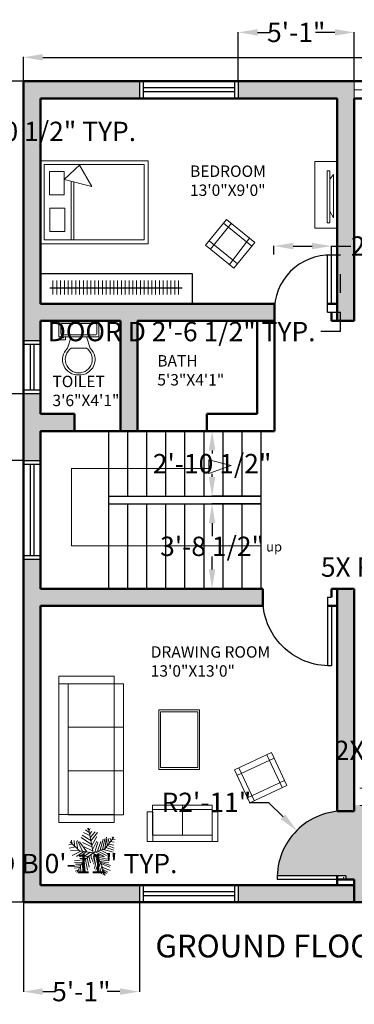
# Model space of a CAD drawing. Units: inches. Extents: x 18 to 9768, y 4 to 3529.
# Tile 4 of 6: x 9249 to 9424, y 3005 to 3523. Entities that reach past the tile are written whole.
import ezdxf

# ---------------------------------------------------------------- set-up
doc = ezdxf.new("R2010")
doc.units = ezdxf.units.IN
doc.header["$MEASUREMENT"] = 0
doc.linetypes.add('ACAD_ISO02W100', pattern=[15, 12, -3])
for name, color, linetype, lineweight in [('A-ANNO-DIMS', 2, 'Continuous', 18), ('A-ANNO-SYMB', 2, 'Continuous', 18), ('A-ANNO-TEXT', 7, 'Continuous', 25), ('A-AREA-IDEN', 7, 'Continuous', 18), ('A-CASE-PATT', 9, 'Continuous', 13), ('A-EQPM', 8, 'Continuous', 18), ('A-FLOR-CASE', 9, 'Continuous', 25), ('A-FLOR-FIXT', 9, 'Continuous', 18), ('A-FLOR-STRS', 7, 'Continuous', 25), ('A-FURN', 8, 'Continuous', 18), ('A-WALL-OVHD', 8, 'ACAD_ISO02W100', 18), ('A-WALL-PATT', 252, 'Continuous', 13), ('L-PLNT', 3, 'Continuous', 18), ('WAL', 7, 'Continuous', 50)]:
    doc.layers.add(name, color=color, linetype=linetype, lineweight=lineweight)
for name, color, linetype, lineweight, true_color in [('A-DOOR', 30, 'Continuous', 25, 0xf8991e), ('A-FLOR-PATT', 254, 'Continuous', 13, 0xddb3d4), ('A-GLAZ', 177, 'Continuous', 25, 0x293189)]:
    doc.layers.add(name, color=color, linetype=linetype, lineweight=lineweight, true_color=true_color)
doc.styles.get("Standard").update_dxf_attribs({"font": 'arial.ttf'})
doc.dimstyles.get("Standard").update_dxf_attribs({"dimtxt": 10.18, "dimasz": 10.18, "dimexe": 0.18, "dimexo": 0.0625, "dimgap": 0.09, "dimtad": 0, "dimtih": 1, "dimtoh": 1, "dimdec": 0, "dimzin": 0, "dimdsep": 46, "dimlunit": 3, "dimtxsty": 'Standard', "dimcen": 0.09, "dimadec": 0, "dimazin": 0, "dimtfac": 1, "dimtdec": 0, "dimtofl": 0, "dimtmove": 0, "dimatfit": 3, "dimfxl": 1, "dimtolj": 1, "dimtzin": 0, "dimarcsym": 0})

# ---------------------------------------------------------------- blocks, each defined once
blk = doc.blocks.new('*U2')
for p, q in [((9.5, -6), (9.5, -2)), ((-10, -8.5), (-8, -8.5)), ((-10, -9.5), (-10, -8.5)), ((-7, -9.5), (-10, -9.5)), ((-8, -8.5), (-8, -8)), ((-7, -8), (-7, -9.5)), ((-4, -8), (-6, -14)), ((4, -8), (6, -14)), ((4, -14), (-4, -14))]:
    blk.add_line(p, q)
blk.add_lwpolyline([(10.5, -8), (10.5, 0), (-10.5, 0), (-10.5, -8)], close=True)
for points in [[(-9.5, -2), (-9.5, -6)], [(8.5, -1), (-8.5, -1)], [(-8.5, -7), (8.5, -7)]]:
    blk.add_lwpolyline(points)
for centre, radius, start, end in [((-8.625, -1.875), 0.8839, 81.8699, 188.1301), ((8.625, -1.875), 0.8839, 351.8699, 98.1301), ((-8.625, -6.125), 0.8839, 171.869898, 278.1301), ((8.625, -6.125), 0.8839, 261.8699, 8.1301), ((-0.4772, -19.9188), 8.0953, 133.01722, 273.38), ((0.0374, -19.8731), 7.127, 124.50543, 269.7), ((-0.0373, -19.8731), 7.127, 270.3, 55.4946), ((0.4773, -19.9188), 8.0953, 266.62, 46.9828)]:
    blk.add_arc(centre, radius, start, end)
blk = doc.blocks.new('*U6')
for p, q in [((-7.288, 39.707), (-21.778, 46.673)), ((-8.737, 47.138), (-17.069, 52.711)), ((-10.186, 53.64), (-13.084, 55.962)), ((0, 0), (-10.5, 57)), ((-9.099, 51.782), (-6.563, 55.962)), ((-7.65, 43.423), (-2.578, 49.46)), ((-5.839, 35.992), (4.667, 48.067)), ((-5.114, 27.632), (10.463, 46.673)), ((-31.5, 4.5), (-52.5, 25.5)), ((-48.585, 21.131), (-49.309, 29.026)), ((-43.513, 28.561), (-42.427, 15.558)), ((-38.442, 26.239), (-34.819, 7.663)), ((-35.544, 28.097), (-24.314, 3.947)), ((-14.533, 2.09), (-30.834, 25.31)), ((-3.665, 19.273), (-27.574, 35.527)), ((-5.114, 28.097), (-24.676, 40.636)), ((-24.314, 23.917), (-2.941, 13.7)), ((-2.941, 16.486), (8.652, 37.85)), ((-1.129, 6.734), (9.014, 26.704)), ((3.942, 1.625), (11.187, 24.381)), ((10.101, 3.483), (17.708, 26.239)), ((16.259, 5.805), (23.142, 31.348)), ((22.055, 7.198), (27.489, 32.277)), ((27, 9), (48, 36)), ((27.127, 9.056), (31.112, 35.992)), ((31.836, 30.883), (32.561, 16.486)), ((35.096, 32.741), (37.27, 22.524)), ((38.719, 34.134), (41.979, 28.561)), ((40.53, 25.775), (48.862, 24.846)), ((43.791, 29.954), (51.036, 30.883)), ((44.153, 36.456), (45.239, 32.741)), ((-47.498, 19.737), (-55.83, 18.344)), ((-40.615, 13.7), (-55.105, 10.913)), ((-33.37, 6.269), (-52.207, 5.34)), ((-28.299, 3.483), (-47.86, -5.805)), ((-21.416, 3.018), (-38.079, -8.128)), ((0, 0), (-31.5, 4.5)), ((-15.982, 2.09), (-30.11, -9.521)), ((0, 0), (-22.5, -19.5)), ((-6.563, 1.161), (-21.416, -8.128)), ((-20.691, 13.7), (-1.129, 4.876)), ((0, 0), (27, 9)), ((0, 0), (18, -22.5)), ((6.478, 1.625), (26.04, -8.592)), ((11.187, 3.483), (30.749, -5.805)), ((18.07, 5.805), (35.096, -3.483)), ((24.229, 7.663), (46.688, 1.625)), ((29.662, 12.307), (48.137, 6.269)), ((33.285, 16.486), (48.862, 10.913)), ((36.183, 19.737), (48.137, 17.88)), ((-17.431, -15.094), (-42.789, -18.809)), ((-24.314, -21.596), (-42.427, -22.06)), ((-22.5, -19.5), (-37.5, -45)), ((-15.257, -12.772), (-30.11, -12.772)), ((-20.691, -18.345), (-17.793, -44.352)), ((-6.563, -5.805), (-19.967, -9.985)), ((-17.069, -15.094), (-12.721, -40.172)), ((-13.446, -11.378), (-8.737, -32.741)), ((-9.461, -8.592), (-6.201, -23.453)), ((-4.752, -3.483), (-3.665, -14.629)), ((2.493, -3.019), (-1.491, -20.202)), ((1.769, -2.555), (24.229, -9.521)), ((5.029, -6.27), (2.131, -25.775)), ((9.014, -11.378), (3.58, -35.992)), ((14.085, -16.951), (6.478, -40.172)), ((7.565, -9.056), (32.198, -14.629)), ((18.07, -22.524), (8.289, -45.745)), ((12.274, -15.094), (36.907, -18.809)), ((16.259, -19.738), (36.183, -22.989)), ((18, -22.5), (27, -52.5)), ((18.433, -22.524), (40.53, -29.026)), ((-28.299, -29.026), (-42.789, -31.348)), ((-30.834, -34.135), (-42.427, -35.528)), ((-34.457, -39.708), (-40.978, -42.494)), ((-26.849, -26.24), (-40.253, -25.775)), ((-32.646, -36.921), (-31.921, -44.352)), ((-29.023, -30.884), (-27.936, -43.887)), ((-25.038, -23.918), (-22.865, -45.281)), ((20.244, -30.419), (15.897, -44.816)), ((19.157, -25.311), (38.719, -33.206)), ((22.78, -37.85), (19.519, -48.532)), ((21.331, -32.741), (39.081, -40.636)), ((22.78, -38.314), (34.372, -44.816)), ((24.591, -43.423), (30.749, -47.603)), ((24.591, -45.745), (23.142, -50.854)), ((26.764, -49.925), (28.213, -50.854))]:
    blk.add_line(p, q)
blk = doc.blocks.new('*D7')
at = {"layer": 'A-ANNO-DIMS', "color": 0, "lineweight": -2, "transparency": 16777216}
for p, q in [((9250.43, 3490.42), (9250.43, 3503.16)), ((9260.61, 3502.98), (9433.71, 3502.98)), ((9624.25, 3502.98), (9451.16, 3502.98)), ((9634.43, 3490.42), (9634.43, 3503.16))]:
    blk.add_line(p, q, dxfattribs=at)
at = {"layer": 'A-ANNO-DIMS', "color": 0, "transparency": 16777216}
for points in [[(9260.61, 3504.67), (9260.61, 3501.28), (9250.43, 3502.98)], [(9624.25, 3504.67), (9624.25, 3501.28), (9634.43, 3502.98)]]:
    blk.add_solid(points, dxfattribs=at)
at = {"layer": 'Defpoints', "color": 0, "transparency": 16777216}
for p in [(9634.43, 3502.98), (9250.43, 3490.36), (9634.43, 3490.36)]:
    blk.add_point(p, dxfattribs=at)
at = {"layer": 'A-ANNO-DIMS', "color": 0, "transparency": 16777216, "insert": (9442.43, 3502.98), "char_height": 10.18, "attachment_point": 5}
blk.add_mtext("\\A1;32'", dxfattribs=at)
blk = doc.blocks.new('*D8')
at = {"layer": 'A-ANNO-DIMS', "color": 0, "lineweight": -2, "transparency": 16777216}
for p, q in [((9250.37, 3490.36), (9231.16, 3490.36)), ((9231.34, 3480.18), (9231.34, 3279.65)), ((9231.34, 3068.54), (9231.34, 3269.07)), ((9250.37, 3058.36), (9231.16, 3058.36))]:
    blk.add_line(p, q, dxfattribs=at)
at = {"layer": 'A-ANNO-DIMS', "color": 0, "transparency": 16777216}
for points in [[(9229.65, 3480.18), (9233.04, 3480.18), (9231.34, 3490.36)], [(9229.65, 3068.54), (9233.04, 3068.54), (9231.34, 3058.36)]]:
    blk.add_solid(points, dxfattribs=at)
at = {"layer": 'Defpoints', "color": 0, "transparency": 16777216}
for p in [(9250.43, 3490.36), (9231.34, 3058.36), (9250.43, 3058.36)]:
    blk.add_point(p, dxfattribs=at)
at = {"layer": 'A-ANNO-DIMS', "color": 0, "transparency": 16777216, "insert": (9231.34, 3274.36), "char_height": 10.18, "attachment_point": 5}
blk.add_mtext("\\A1;36'", dxfattribs=at)
blk = doc.blocks.new('WINDOW-48')
for p, q in [((0, 0), (0, 9)), ((2, 0), (2, 9)), ((2, 5.5), (50, 5.5)), ((50, 0), (50, 9)), ((52, 0), (52, 9)), ((2, 3.5), (50, 3.5))]:
    blk.add_line(p, q)
blk = doc.blocks.new('WINDOW-24')
for p, q in [((9, 28), (0, 28)), ((9, 26), (0, 26)), ((3.5, 26), (3.5, 2)), ((5.5, 26), (5.5, 2)), ((9, 2), (0, 2)), ((9, 0), (0, 0))]:
    blk.add_line(p, q)
blk = doc.blocks.new('DOOR-36-W9')
for p, q in [((2, 36.01), (0, 36.01)), ((0, 31.51), (0, 0.01)), ((2, 36.01), (2, 0.01))]:
    blk.add_line(p, q)
blk.add_arc((1, 35.01), 35.01, 268.3634, 1.6366)
blk = doc.blocks.new('DOOR-30-W9')
for p, q in [((25.52, 30.02), (0.02, 30.02)), ((30.02, 28.02), (0.02, 28.02)), ((30.02, 28.02), (30.02, 30.02))]:
    blk.add_line(p, q)
blk.add_arc((29.02, 29.02), 29.02, 178.0251, 271.9749)
blk = doc.blocks.new('*D35')
at = {"layer": 'A-ANNO-DIMS', "color": 0, "lineweight": -2, "transparency": 16777216}
for p, q in [((9412.5, 3399.14), (9417.16, 3399.14)), ((9416.98, 3388.96), (9416.98, 3379.04)), ((9412.5, 3368.86), (9417.16, 3368.86)), ((9416.98, 3368.86), (9416.98, 3358.68)), ((9416.98, 3358.68), (9406.8, 3358.68))]:
    blk.add_line(p, q, dxfattribs=at)
at = {"layer": 'A-ANNO-DIMS', "color": 0, "transparency": 16777216}
for points in [[(9415.28, 3388.96), (9418.67, 3388.96), (9416.98, 3399.14)], [(9415.28, 3379.04), (9418.67, 3379.04), (9416.98, 3368.86)]]:
    blk.add_solid(points, dxfattribs=at)
at = {"layer": 'Defpoints', "color": 0, "transparency": 16777216}
for p in [(9412.43, 3399.14), (9412.43, 3368.86), (9416.98, 3368.86)]:
    blk.add_point(p, dxfattribs=at)
at = {"layer": 'A-ANNO-DIMS', "color": 0, "transparency": 16777216, "insert": (9333.65, 3358.68), "char_height": 10.18, "attachment_point": 5}
blk.add_mtext('\\A1;DOOR D 2\'-6 1/2" TYP.', dxfattribs=at)
blk = doc.blocks.new('*D36')
at = {"layer": 'A-ANNO-DIMS', "color": 0, "lineweight": -2, "transparency": 16777216}
for p, q in [((9382.16, 3399.2), (9382.16, 3403.86)), ((9392.34, 3403.68), (9402.25, 3403.68)), ((9412.43, 3399.2), (9412.43, 3403.86)), ((9412.43, 3403.68), (9422.61, 3403.68))]:
    blk.add_line(p, q, dxfattribs=at)
at = {"layer": 'A-ANNO-DIMS', "color": 0, "transparency": 16777216}
for points in [[(9392.34, 3405.38), (9392.34, 3401.98), (9382.16, 3403.68)], [(9402.25, 3405.38), (9402.25, 3401.98), (9412.43, 3403.68)]]:
    blk.add_solid(points, dxfattribs=at)
at = {"layer": 'Defpoints', "color": 0, "transparency": 16777216}
for p in [(9382.16, 3399.14), (9412.43, 3403.68), (9412.43, 3399.14)]:
    blk.add_point(p, dxfattribs=at)
at = {"layer": 'A-ANNO-DIMS', "color": 0, "transparency": 16777216, "insert": (9465.68, 3403.68), "char_height": 10.18, "attachment_point": 5}
blk.add_mtext('\\A1;2\'-6 1/2" TYP.', dxfattribs=at)
blk = doc.blocks.new('*D49')
at = {"layer": 'A-ANNO-DIMS', "color": 0, "lineweight": -2, "transparency": 16777216}
for p, q in [((9121.17, 3464.01), (9110.99, 3464.01)), ((9131.35, 3465.54), (9131.35, 3463.83)), ((9141.99, 3465.54), (9141.99, 3463.83)), ((9152.17, 3464.01), (9162.35, 3464.01))]:
    blk.add_line(p, q, dxfattribs=at)
at = {"layer": 'A-ANNO-DIMS', "color": 0, "transparency": 16777216}
for points in [[(9121.17, 3465.71), (9121.17, 3462.32), (9131.35, 3464.01)], [(9152.17, 3465.71), (9152.17, 3462.32), (9141.99, 3464.01)]]:
    blk.add_solid(points, dxfattribs=at)
at = {"layer": 'Defpoints', "color": 0, "transparency": 16777216}
for p in [(9131.35, 3465.61), (9141.99, 3465.61), (9141.99, 3464.01)]:
    blk.add_point(p, dxfattribs=at)
at = {"layer": 'A-ANNO-DIMS', "color": 0, "transparency": 16777216, "insert": (9237.11, 3464.01), "char_height": 10.18, "attachment_point": 5}
blk.add_mtext('\\A1;LAMP B 0\'-10 1/2" TYP.', dxfattribs=at)
blk = doc.blocks.new('*D55')
at = {"layer": 'A-ANNO-DIMS', "color": 0, "lineweight": -2, "transparency": 16777216}
for p, q in [((9114.26, 3078.78), (9104.08, 3078.78)), ((9124.44, 3080.36), (9124.44, 3078.6)), ((9135.38, 3080.36), (9135.38, 3078.6)), ((9145.56, 3078.78), (9155.74, 3078.78))]:
    blk.add_line(p, q, dxfattribs=at)
at = {"layer": 'A-ANNO-DIMS', "color": 0, "transparency": 16777216}
for points in [[(9114.26, 3080.48), (9114.26, 3077.09), (9124.44, 3078.78)], [(9145.56, 3080.48), (9145.56, 3077.09), (9135.38, 3078.78)]]:
    blk.add_solid(points, dxfattribs=at)
at = {"layer": 'Defpoints', "color": 0, "transparency": 16777216}
for p in [(9124.44, 3080.42), (9135.38, 3080.42), (9135.38, 3078.78)]:
    blk.add_point(p, dxfattribs=at)
at = {"layer": 'A-ANNO-DIMS', "color": 0, "transparency": 16777216, "insert": (9245.48, 3078.78), "char_height": 10.18, "attachment_point": 5}
blk.add_mtext('\\A1;NIGHTSTAND B 0\'-11" TYP.', dxfattribs=at)
blk = doc.blocks.new('*D63')
at = {"layer": 'A-ANNO-DIMS', "color": 0, "lineweight": -2, "transparency": 16777216}
for p, q in [((9375.37, 3306.36), (9349.5, 3306.36)), ((9349.68, 3296.18), (9349.68, 3294.53)), ((9349.68, 3282.18), (9349.68, 3283.83)), ((9375.37, 3272), (9349.5, 3272))]:
    blk.add_line(p, q, dxfattribs=at)
at = {"layer": 'A-ANNO-DIMS', "color": 0, "transparency": 16777216}
for points in [[(9347.99, 3296.18), (9351.38, 3296.18), (9349.68, 3306.36)], [(9347.99, 3282.18), (9351.38, 3282.18), (9349.68, 3272)]]:
    blk.add_solid(points, dxfattribs=at)
at = {"layer": 'Defpoints', "color": 0, "transparency": 16777216}
for p in [(9349.68, 3306.36), (9375.43, 3306.36), (9375.43, 3272)]:
    blk.add_point(p, dxfattribs=at)
at = {"layer": 'A-ANNO-DIMS', "color": 0, "transparency": 16777216, "insert": (9349.68, 3289.18), "char_height": 10.18, "attachment_point": 5}
blk.add_mtext('\\A1;2\'-10 1/2"', dxfattribs=at)
blk = doc.blocks.new('*D64')
at = {"layer": 'A-ANNO-DIMS', "color": 0, "lineweight": -2, "transparency": 16777216}
for p, q in [((9375.37, 3268), (9349.5, 3268)), ((9349.68, 3257.82), (9349.68, 3251.04)), ((9349.68, 3233.54), (9349.68, 3240.32)), ((9375.37, 3223.36), (9349.5, 3223.36))]:
    blk.add_line(p, q, dxfattribs=at)
at = {"layer": 'A-ANNO-DIMS', "color": 0, "transparency": 16777216}
for points in [[(9347.99, 3257.82), (9351.38, 3257.82), (9349.68, 3268)], [(9347.99, 3233.54), (9351.38, 3233.54), (9349.68, 3223.36)]]:
    blk.add_solid(points, dxfattribs=at)
at = {"layer": 'Defpoints', "color": 0, "transparency": 16777216}
for p in [(9349.68, 3268), (9375.43, 3268), (9375.43, 3223.36)]:
    blk.add_point(p, dxfattribs=at)
at = {"layer": 'A-ANNO-DIMS', "color": 0, "transparency": 16777216, "insert": (9349.68, 3245.68), "char_height": 10.18, "attachment_point": 5}
blk.add_mtext('\\A1;3\'-8 1/2"', dxfattribs=at)
blk = doc.blocks.new('*D65')
at = {"layer": 'A-ANNO-DIMS', "color": 0, "lineweight": -2, "transparency": 16777216}
for p, q in [((9250.43, 3058.3), (9250.43, 3011.2)), ((9311.43, 3058.3), (9311.43, 3011.2)), ((9260.61, 3011.38), (9267.31, 3011.38)), ((9301.25, 3011.38), (9294.55, 3011.38))]:
    blk.add_line(p, q, dxfattribs=at)
at = {"layer": 'A-ANNO-DIMS', "color": 0, "transparency": 16777216}
for points in [[(9260.61, 3013.08), (9260.61, 3009.68), (9250.43, 3011.38)], [(9301.25, 3013.08), (9301.25, 3009.68), (9311.43, 3011.38)]]:
    blk.add_solid(points, dxfattribs=at)
at = {"layer": 'Defpoints', "color": 0, "transparency": 16777216}
for p in [(9250.43, 3058.36), (9311.43, 3058.36), (9311.43, 3011.38)]:
    blk.add_point(p, dxfattribs=at)
at = {"layer": 'A-ANNO-DIMS', "color": 0, "transparency": 16777216, "insert": (9280.93, 3011.38), "char_height": 10.18, "attachment_point": 5}
blk.add_mtext('\\A1;5\'-1"', dxfattribs=at)
blk = doc.blocks.new('*D72')
at = {"layer": 'A-ANNO-DIMS', "color": 0, "lineweight": -2, "transparency": 16777216}
for p, q in [((9414.25, 3516.11), (9404.07, 3516.11)), ((9424.43, 3490.42), (9424.43, 3516.29)), ((9472.43, 3490.42), (9472.43, 3516.29)), ((9482.61, 3516.11), (9492.79, 3516.11))]:
    blk.add_line(p, q, dxfattribs=at)
at = {"layer": 'A-ANNO-DIMS', "color": 0, "transparency": 16777216}
for points in [[(9414.25, 3517.81), (9414.25, 3514.41), (9424.43, 3516.11)], [(9482.61, 3517.81), (9482.61, 3514.41), (9472.43, 3516.11)]]:
    blk.add_solid(points, dxfattribs=at)
at = {"layer": 'Defpoints', "color": 0, "transparency": 16777216}
for p in [(9472.43, 3516.11), (9424.43, 3490.36), (9472.43, 3490.36)]:
    blk.add_point(p, dxfattribs=at)
at = {"layer": 'A-ANNO-DIMS', "color": 0, "transparency": 16777216, "insert": (9448.43, 3516.11), "char_height": 10.18, "attachment_point": 5}
blk.add_mtext('\\A1;4\'-0"', dxfattribs=at)
blk = doc.blocks.new('*D73')
at = {"layer": 'A-ANNO-DIMS', "color": 0, "lineweight": -2, "transparency": 16777216}
for p, q in [((9363.42, 3490.42), (9363.42, 3516.29)), ((9373.6, 3516.11), (9380.31, 3516.11)), ((9414.25, 3516.11), (9407.55, 3516.11)), ((9424.43, 3490.42), (9424.43, 3516.29))]:
    blk.add_line(p, q, dxfattribs=at)
at = {"layer": 'A-ANNO-DIMS', "color": 0, "transparency": 16777216}
for points in [[(9373.6, 3517.81), (9373.6, 3514.41), (9363.42, 3516.11)], [(9414.25, 3517.81), (9414.25, 3514.41), (9424.43, 3516.11)]]:
    blk.add_solid(points, dxfattribs=at)
at = {"layer": 'Defpoints', "color": 0, "transparency": 16777216}
for p in [(9424.43, 3516.11), (9363.42, 3490.36), (9424.43, 3490.36)]:
    blk.add_point(p, dxfattribs=at)
at = {"layer": 'A-ANNO-DIMS', "color": 0, "transparency": 16777216, "insert": (9393.93, 3516.11), "char_height": 10.18, "attachment_point": 5}
blk.add_mtext('\\A1;5\'-1"', dxfattribs=at)
blk = doc.blocks.new('*D78')
at = {"layer": 'A-ANNO-DIMS', "color": 0, "lineweight": -2, "transparency": 16777216}
for p, q in [((9250.37, 3325.86), (9224.5, 3325.86)), ((9224.68, 3315.68), (9224.68, 3313.56)), ((9224.68, 3301.04), (9224.68, 3303.16)), ((9250.37, 3290.86), (9224.5, 3290.86))]:
    blk.add_line(p, q, dxfattribs=at)
at = {"layer": 'A-ANNO-DIMS', "color": 0, "transparency": 16777216}
for points in [[(9222.99, 3315.68), (9226.38, 3315.68), (9224.68, 3325.86)], [(9222.99, 3301.04), (9226.38, 3301.04), (9224.68, 3290.86)]]:
    blk.add_solid(points, dxfattribs=at)
at = {"layer": 'Defpoints', "color": 0, "transparency": 16777216}
for p in [(9224.68, 3325.86), (9250.43, 3325.86), (9250.43, 3290.86)]:
    blk.add_point(p, dxfattribs=at)
at = {"layer": 'A-ANNO-DIMS', "color": 0, "transparency": 16777216, "insert": (9224.68, 3308.36), "char_height": 10.18, "attachment_point": 5}
blk.add_mtext('\\A1;2\'-11"', dxfattribs=at)
blk = doc.blocks.new('*D82')
at = {"layer": 'A-ANNO-DIMS', "color": 0, "lineweight": -2, "transparency": 16777216}
for p, q in [((9517.84, 3173.21), (9518.02, 3173.21)), ((9517.93, 3173.12), (9517.93, 3173.3)), ((9483.02, 3138.3), (9490.22, 3145.5)), ((9472.84, 3138.3), (9483.02, 3138.3))]:
    blk.add_line(p, q, dxfattribs=at)
at = {"layer": 'A-ANNO-DIMS', "color": 0, "transparency": 16777216}
blk.add_solid([(9489.02, 3146.7), (9491.42, 3144.3), (9497.42, 3152.7)], dxfattribs=at)
at = {"layer": 'Defpoints', "color": 0, "transparency": 16777216}
for p in [(9517.93, 3173.21), (9497.42, 3152.7)]:
    blk.add_point(p, dxfattribs=at)
at = {"layer": 'A-ANNO-DIMS', "color": 0, "transparency": 16777216, "insert": (9443.32, 3138.3), "char_height": 10.18, "attachment_point": 5}
blk.add_mtext('\\A1;2X R2\'-5"', dxfattribs=at)
blk = doc.blocks.new('*D84')
at = {"layer": 'A-ANNO-DIMS', "color": 0, "lineweight": -2, "transparency": 16777216}
for p, q in [((9499.78, 3262.71), (9499.96, 3262.71)), ((9499.87, 3262.62), (9499.87, 3262.8)), ((9499.49, 3234.76), (9499.63, 3244.93)), ((9489.31, 3234.76), (9499.49, 3234.76))]:
    blk.add_line(p, q, dxfattribs=at)
at = {"layer": 'A-ANNO-DIMS', "color": 0, "transparency": 16777216}
blk.add_solid([(9497.93, 3244.96), (9501.32, 3244.91), (9499.77, 3255.11)], dxfattribs=at)
at = {"layer": 'Defpoints', "color": 0, "transparency": 16777216}
for p in [(9499.87, 3262.71), (9499.77, 3255.11)]:
    blk.add_point(p, dxfattribs=at)
at = {"layer": 'A-ANNO-DIMS', "color": 0, "transparency": 16777216, "insert": (9448.02, 3234.76), "char_height": 10.18, "attachment_point": 5}
blk.add_mtext('\\A1;5X R0\'-7 1/2"', dxfattribs=at)
blk = doc.blocks.new('*D87')
at = {"layer": 'A-ANNO-DIMS', "color": 0, "lineweight": -2, "transparency": 16777216}
for p, q in [((9369.14, 3110.97), (9379.32, 3110.97)), ((9379.32, 3110.97), (9386.98, 3103.32)), ((9418.84, 3071.36), (9419.02, 3071.36)), ((9418.93, 3071.27), (9418.93, 3071.45))]:
    blk.add_line(p, q, dxfattribs=at)
at = {"layer": 'A-ANNO-DIMS', "color": 0, "transparency": 16777216}
blk.add_solid([(9388.18, 3104.52), (9385.78, 3102.12), (9394.17, 3096.12)], dxfattribs=at)
at = {"layer": 'Defpoints', "color": 0, "transparency": 16777216}
for p in [(9394.17, 3096.12), (9418.93, 3071.36)]:
    blk.add_point(p, dxfattribs=at)
at = {"layer": 'A-ANNO-DIMS', "color": 0, "transparency": 16777216, "insert": (9346.69, 3110.97), "char_height": 10.18, "attachment_point": 5}
blk.add_mtext('\\A1;R2\'-11"', dxfattribs=at)

msp = doc.modelspace()

# ---------------------------------------------------------------- hatches: boundary and pattern name
at = {"layer": 'A-CASE-PATT'}
h = msp.add_hatch(dxfattribs=at)
h.set_pattern_fill('ANSI31', color=256, scale=16, angle=45, style=0)
h.paths.add_polyline_path([(9265.9, 3378.15), (9333.9, 3378.15), (9333.9, 3385.6), (9265.9, 3385.6)])
at = {"layer": 'A-FLOR-PATT'}
h = msp.add_hatch(color=256, dxfattribs=at)
h.dxf.hatch_style = 1
h.paths.add_polyline_path([(9583.28, 3058.36), (9532.08, 3058.36), (9532.08, 3047.74), (9583.28, 3047.74)])
h.paths.add_polyline_path([(9583.28, 3047.74), (9532.08, 3047.74), (9532.08, 3037.13), (9583.28, 3037.13)])
h.paths.add_polyline_path([(9615.06, 3076.24), (9634.43, 3076.24), (9634.43, 3109.36), (9625.43, 3109.36), (9454.43, 3109.36), (9424.43, 3109.36), (9424.43, 3106.36), (9417.93, 3106.36, 0.397579), (9383.93, 3072.36), (9419.93, 3072.36), (9419.93, 3070.36), (9424.43, 3070.36), (9424.43, 3067.36), (9424.43, 3058.36), (9615.06, 3058.36)])
h.paths.add_polyline_path([(9509.39, 3070.22), (9559.29, 3070.22), (9559.29, 3092.61), (9509.39, 3092.61)], flags=24)
at = {"layer": 'A-WALL-PATT'}
h = msp.add_hatch(color=256, dxfattribs=at)
h.dxf.hatch_style = 1
h.paths.add_polyline_path([(9424.43, 3490.36), (9363.42, 3490.36), (9363.42, 3481.36), (9373.43, 3481.36), (9382.43, 3481.36), (9415.43, 3481.36), (9415.43, 3373.36), (9415.43, 3364.36), (9424.43, 3364.36), (9424.43, 3373.36), (9424.43, 3481.36)])
h.paths.add_polyline_path([(9527.43, 3490.36), (9472.43, 3490.36), (9472.43, 3481.36), (9472.43, 3373.36), (9472.43, 3364.36), (9481.43, 3364.36), (9481.43, 3373.36), (9481.43, 3481.36), (9527.43, 3481.36)])
h.paths.add_polyline_path([(9311.42, 3490.36), (9250.43, 3490.36), (9250.43, 3353.86), (9259.43, 3353.86), (9259.43, 3364.36), (9301.43, 3364.36), (9301.43, 3315.36), (9301.43, 3306.36), (9310.43, 3306.36), (9310.43, 3315.36), (9310.43, 3364.36), (9382.43, 3364.36), (9382.43, 3368.86, -0.017236), (9382.43, 3370.86), (9382.43, 3373.36), (9259.43, 3373.36), (9259.43, 3481.36), (9311.42, 3481.36)])
h.paths.add_polyline_path([(9376.43, 3216.86, -0.014283), (9376.43, 3218.86), (9376.43, 3223.36), (9259.43, 3223.36), (9259.43, 3238.86), (9250.43, 3238.86), (9250.43, 3058.36), (9311.43, 3058.36), (9311.43, 3067.36), (9259.43, 3067.36), (9259.43, 3214.36), (9376.43, 3214.36)])
h.paths.add_polyline_path([(9382.43, 3364.36), (9373.43, 3364.36), (9373.43, 3315.36), (9347, 3315.36), (9347, 3306.36), (9382.43, 3306.36)], flags=0)
h.paths.add_polyline_path([(9277.41, 3315.36), (9259.43, 3315.36), (9259.43, 3325.86), (9250.43, 3325.86), (9250.43, 3290.86), (9259.43, 3290.86), (9259.43, 3306.36), (9277.41, 3306.36)])
h.paths.add_polyline_path([(9424.43, 3214.36), (9424.43, 3223.36), (9415.43, 3223.36), (9415.43, 3214.36), (9415.43, 3106.36), (9417.93, 3106.36, -0.014283), (9419.93, 3106.36), (9424.43, 3106.36), (9424.43, 3109.36), (9424.43, 3118.36)])
h.paths.add_polyline_path([(9463.43, 3214.36), (9463.43, 3223.36), (9454.43, 3223.36), (9454.43, 3214.36), (9454.43, 3118.36), (9454.43, 3109.36), (9548.43, 3109.36), (9548.43, 3118.36), (9523.43, 3118.36), (9523.43, 3144.21), (9518.93, 3144.21, -0.017236), (9516.93, 3144.21), (9514.43, 3144.21), (9514.43, 3118.36), (9463.43, 3118.36)])
h.paths.add_polyline_path([(9523.43, 3214.36), (9523.43, 3223.36), (9514.43, 3223.36), (9514.43, 3214.36), (9514.43, 3177.21), (9523.43, 3177.21)], flags=17)
h.paths.add_polyline_path([(9514.43, 3193.54), (9463.43, 3193.54), (9463.43, 3184.54), (9514.43, 3184.54)], flags=17)
h.paths.add_polyline_path([(9634.43, 3267.86), (9625.43, 3267.86), (9625.43, 3223.36), (9569.35, 3223.36), (9569.35, 3214.36), (9625.43, 3214.36), (9625.43, 3118.36), (9600.43, 3118.36), (9600.43, 3109.36), (9625.43, 3109.36), (9634.43, 3109.36)])
h.paths.add_polyline_path([(9634.43, 3490.36), (9579.43, 3490.36), (9579.43, 3481.36), (9625.43, 3481.36), (9625.43, 3373.36), (9520.43, 3373.36), (9520.43, 3370.86, -0.014283), (9520.43, 3368.86), (9520.43, 3364.36), (9625.43, 3364.36), (9625.43, 3319.86), (9634.43, 3319.86)])
h.paths.add_polyline_path([(9424.43, 3067.36), (9415.43, 3067.36), (9363.43, 3067.36), (9363.43, 3058.36), (9424.43, 3058.36)])

# ---------------------------------------------------------------- linework, layer by layer
at = {"layer": 'A-ANNO-SYMB'}
for p, q in [((9347.9, 3286.72), (9347.9, 3291.2)), ((9347.9, 3291.2), (9347.9, 3284.01)), ((9359.67, 3288.29), (9347.9, 3291.2)), ((9275.67, 3245.9), (9275.67, 3286.72)), ((9275.67, 3286.72), (9347.9, 3286.72)), ((9347.9, 3284.01), (9359.67, 3288.29)), ((9375.43, 3245.9), (9275.67, 3245.9))]:
    msp.add_line(p, q, dxfattribs=at)
at = {"layer": 'A-DOOR'}
for p, q in [((9419.93, 3072.36), (9383.93, 3072.36)), ((9419.93, 3072.36), (9419.93, 3070.36)), ((9419.93, 3070.36), (9383.93, 3070.36))]:
    msp.add_line(p, q, dxfattribs=at)
msp.add_arc((9418.93, 3071.36), 35.01, 88.3634, 181.6366, dxfattribs=at)
at = {"layer": 'A-EQPM'}
for p, q in [((9411.59, 3438.86), (9413.44, 3441.42)), ((9413.44, 3441.42), (9413.44, 3418.55)), ((9413.44, 3418.55), (9411.59, 3422.03))]:
    msp.add_line(p, q, dxfattribs=at)
for points in [[(9415.43, 3448.09), (9415.43, 3448.09), (9403.64, 3448.09), (9403.64, 3448.09), (9403.64, 3413.12), (9403.64, 3413.12), (9415.43, 3413.12), (9415.43, 3413.12)], [(9410.26, 3443.27), (9410.26, 3443.27), (9411.59, 3443.27), (9411.59, 3443.27), (9411.59, 3415.98), (9411.59, 3415.98), (9410.26, 3415.98), (9410.26, 3415.98)]]:
    msp.add_lwpolyline(points, close=True, dxfattribs=at)
at = {"layer": 'A-FLOR-CASE'}
for p, q in [((9259.43, 3389.19), (9339.22, 3389.19)), ((9339.22, 3389.19), (9339.22, 3373.36)), ((9264.32, 3381.75), (9333.92, 3381.75))]:
    msp.add_line(p, q, dxfattribs=at)
at = {"layer": 'A-FLOR-STRS'}
for p, q in [((9295.43, 3223.36), (9295.43, 3306.36)), ((9305.43, 3272), (9305.43, 3306.36)), ((9315.43, 3272), (9315.43, 3306.36)), ((9325.43, 3272), (9325.43, 3306.36)), ((9335.43, 3272), (9335.43, 3306.36)), ((9345.43, 3272), (9345.43, 3306.36)), ((9355.43, 3272), (9355.43, 3306.36)), ((9365.43, 3272), (9365.43, 3306.36)), ((9375.43, 3223.36), (9375.43, 3306.36)), ((9295.43, 3272), (9375.43, 3272)), ((9295.43, 3268), (9375.43, 3268)), ((9305.43, 3223.36), (9305.43, 3268)), ((9315.43, 3223.36), (9315.43, 3268)), ((9325.43, 3223.36), (9325.43, 3268)), ((9335.43, 3223.36), (9335.43, 3268)), ((9345.43, 3223.36), (9345.43, 3268)), ((9355.43, 3223.36), (9355.43, 3268)), ((9365.43, 3223.36), (9365.43, 3268))]:
    msp.add_line(p, q, dxfattribs=at)
at = {"layer": 'A-FURN'}
for p, q in [((9280.23, 3446.59), (9271.87, 3438.64)), ((9286.39, 3434.98), (9279.88, 3446.26)), ((9271.87, 3438.64), (9286.39, 3434.98)), ((9275.58, 3437.71), (9275.58, 3406.93)), ((9277.04, 3437.34), (9277.04, 3406.93)), ((9359.8, 3415.64), (9348.79, 3402.07)), ((9355.66, 3415.7), (9370.59, 3403.59)), ((9348.13, 3406.42), (9363.05, 3394.3)), ((9369.41, 3407.84), (9358.84, 3393.91)), ((9298.27, 3173.26), (9298.27, 3104.54)), ((9273.97, 3150.46), (9303.09, 3150.46)), ((9378.46, 3136.01), (9386.53, 3118.76)), ((9362.72, 3125.14), (9382.24, 3134.28)), ((9273.97, 3127.57), (9303.09, 3127.57)), ((9363.77, 3129.13), (9371.85, 3111.88)), ((9387.73, 3122.54), (9368.22, 3113.41)), ((9334.09, 3109.43), (9334.09, 3093.67)), ((9318.42, 3107.22), (9349.76, 3107.22))]:
    msp.add_line(p, q, dxfattribs=at)
for points in [[(9259.43, 3448.59), (9316.01, 3448.59), (9316.01, 3404.93), (9259.43, 3404.93)], [(9261.43, 3446.59), (9261.43, 3446.59), (9314.01, 3446.59), (9314.01, 3446.59), (9314.01, 3406.93), (9314.01, 3406.93), (9261.43, 3406.93), (9261.43, 3406.93)], [(9264.1, 3442.89), (9264.1, 3442.89), (9271.87, 3442.89), (9271.87, 3442.89), (9271.87, 3430.59), (9271.87, 3430.59), (9264.1, 3430.59), (9264.1, 3430.59)], [(9264.39, 3423.7), (9264.39, 3423.7), (9272.16, 3423.7), (9272.16, 3423.7), (9272.16, 3411.4), (9272.16, 3411.4), (9264.39, 3411.4), (9264.39, 3411.4)], [(9357.27, 3417.69), (9357.27, 3417.69), (9372.2, 3405.58), (9372.2, 3405.58), (9361.19, 3392.01), (9361.19, 3392.01), (9346.26, 3404.12), (9346.26, 3404.12)], [(9269.15, 3173.26), (9269.15, 3173.26), (9298.27, 3173.26), (9298.27, 3173.26), (9298.27, 3177.35), (9298.27, 3177.35), (9269.15, 3177.35), (9269.15, 3177.35)], [(9273.97, 3173.26), (9273.97, 3173.26), (9269.15, 3173.26), (9269.15, 3173.26), (9269.15, 3104.54), (9269.15, 3104.54), (9273.97, 3104.54), (9273.97, 3104.54)], [(9303.09, 3173.26), (9303.09, 3173.26), (9273.97, 3173.26), (9273.97, 3173.26), (9273.97, 3104.48), (9273.97, 3104.48), (9303.09, 3104.48), (9303.09, 3104.48)], [(9321.63, 3159.59), (9321.63, 3159.59), (9343.11, 3159.59), (9343.11, 3159.59), (9343.11, 3128.29), (9343.11, 3128.29), (9321.63, 3128.29), (9321.63, 3128.29)], [(9322.63, 3158.59), (9342.11, 3158.59), (9342.11, 3129.29), (9322.63, 3129.29)], [(9361.38, 3128.02), (9361.38, 3128.02), (9380.89, 3137.15), (9380.89, 3137.15), (9388.97, 3119.9), (9388.97, 3119.9), (9369.46, 3110.76), (9369.46, 3110.76)], [(9318.42, 3109.43), (9318.42, 3109.43), (9349.76, 3109.43), (9349.76, 3109.43), (9349.76, 3093.67), (9349.76, 3093.67), (9318.42, 3093.67), (9318.42, 3093.67)], [(9269.15, 3100.45), (9269.15, 3100.45), (9298.27, 3100.45), (9298.27, 3100.45), (9298.27, 3104.54), (9298.27, 3104.54), (9269.15, 3104.54), (9269.15, 3104.54)], [(9318.51, 3090.37), (9318.51, 3090.37), (9315.53, 3090.37), (9315.53, 3090.37), (9315.53, 3106.03), (9315.53, 3106.03), (9318.51, 3106.03), (9318.51, 3106.03)], [(9352.74, 3090.37), (9352.74, 3090.37), (9349.76, 3090.37), (9349.76, 3090.37), (9349.76, 3106.03), (9349.76, 3106.03), (9352.74, 3106.03), (9352.74, 3106.03)], [(9349.76, 3093.67), (9349.76, 3093.67), (9318.51, 3093.67), (9318.51, 3093.67), (9318.51, 3090.37), (9318.51, 3090.37), (9349.76, 3090.37), (9349.76, 3090.37)]]:
    msp.add_lwpolyline(points, close=True, dxfattribs=at)
at = {"layer": 'A-WALL-OVHD'}
for p, q in [((9424.43, 3481.36), (9424.43, 3490.36)), ((9424.43, 3485.86), (9472.43, 3485.86)), ((9454.43, 3118.36), (9424.43, 3118.36)), ((9454.43, 3109.36), (9424.43, 3109.36))]:
    msp.add_line(p, q, dxfattribs=at)
at = {"layer": 'WAL'}
for p, q in [((9250.43, 3058.36), (9250.43, 3490.36)), ((9250.43, 3490.36), (9634.43, 3490.36)), ((9259.43, 3481.36), (9373.43, 3481.36)), ((9259.43, 3373.36), (9259.43, 3481.36)), ((9373.43, 3481.36), (9382.43, 3481.36)), ((9382.43, 3481.36), (9415.43, 3481.36)), ((9415.43, 3373.36), (9415.43, 3481.36)), ((9424.43, 3373.36), (9424.43, 3481.36)), ((9424.43, 3481.36), (9472.43, 3481.36)), ((9259.43, 3373.36), (9382.63, 3373.36)), ((9382.43, 3373.36), (9382.43, 3364.36)), ((9382.43, 3373.36), (9382.43, 3364.36)), ((9382.43, 3373.36), (9382.43, 3364.36)), ((9410.43, 3373.36), (9415.43, 3373.36)), ((9415.43, 3373.36), (9415.43, 3364.36)), ((9424.43, 3373.36), (9424.43, 3364.36)), ((9412.43, 3368.86), (9412.43, 3364.36)), ((9259.43, 3364.36), (9301.43, 3364.36)), ((9259.43, 3315.36), (9259.43, 3364.36)), ((9301.43, 3315.36), (9301.43, 3364.36)), ((9310.43, 3315.36), (9310.43, 3364.36)), ((9310.43, 3364.36), (9382.43, 3364.36)), ((9373.43, 3315.36), (9373.43, 3364.36)), ((9382.43, 3306.36), (9382.43, 3364.36)), ((9412.43, 3364.36), (9415.43, 3364.36)), ((9415.43, 3364.36), (9424.43, 3364.36)), ((9259.43, 3315.36), (9277.41, 3315.36)), ((9277.41, 3315.36), (9277.41, 3306.36)), ((9301.43, 3315.36), (9301.43, 3306.36)), ((9310.43, 3315.36), (9310.43, 3306.36)), ((9347, 3315.36), (9373.43, 3315.36)), ((9347, 3315.36), (9347, 3306.36)), ((9259.43, 3306.36), (9310.43, 3306.36)), ((9259.43, 3223.36), (9259.43, 3306.36)), ((9310.43, 3306.36), (9347, 3306.36)), ((9347, 3306.36), (9382.43, 3306.36)), ((9376.43, 3223.36), (9259.43, 3223.36)), ((9376.43, 3214.36), (9376.43, 3223.36)), ((9412.43, 3218.86), (9412.43, 3223.36)), ((9424.43, 3223.36), (9412.43, 3223.36)), ((9415.43, 3214.36), (9415.43, 3223.36)), ((9424.43, 3214.36), (9424.43, 3223.36)), ((9259.43, 3067.36), (9259.43, 3214.36)), ((9376.59, 3214.36), (9259.43, 3214.36)), ((9415.43, 3214.36), (9410.43, 3214.36)), ((9415.43, 3106.2), (9415.43, 3214.36)), ((9424.43, 3118.36), (9424.43, 3214.36)), ((9424.43, 3109.36), (9424.43, 3118.36)), ((9424.43, 3106.36), (9424.43, 3109.36)), ((9424.43, 3106.36), (9415.43, 3106.36)), ((9415.43, 3067.36), (9415.43, 3072.36)), ((9415.43, 3067.36), (9259.43, 3067.36)), ((9424.43, 3070.36), (9415.43, 3070.36)), ((9424.43, 3067.36), (9415.43, 3067.36)), ((9424.43, 3067.36), (9424.43, 3070.36)), ((9424.43, 3067.36), (9424.43, 3058.36)), ((9634.43, 3058.36), (9250.43, 3058.36))]:
    msp.add_line(p, q, dxfattribs=at)

# ---------------------------------------------------------------- block references
at = {"layer": 'A-DOOR', "rotation": 269.9999999999958}
msp.add_blockref('DOOR-30-W9', (9382.42, 3398.88), dxfattribs=at)
at = {"layer": 'A-DOOR', "extrusion": (0, 0, -1), "zscale": -1}
msp.add_blockref('DOOR-36-W9', (-9412.43, 3182.85), dxfattribs=at)
at = {"layer": 'A-FLOR-FIXT'}
msp.add_blockref('*U2', (9279.58, 3363.89), dxfattribs=at)
at = {"layer": 'A-GLAZ'}
for p, rotation in [((9363.42, 3490.36), 180), ((9250.43, 3290.86), 269.999999999992), ((9363.43, 3067.36), 180)]:
    msp.add_blockref('WINDOW-48', p, dxfattribs=dict(at, rotation=rotation))
msp.add_blockref('WINDOW-24', (9250.43, 3325.86), dxfattribs=at)
at = {"layer": 'L-PLNT', "xscale": 0.2283434584619827, "yscale": 0.2283434584619827, "zscale": 0.2283434584619827}
msp.add_blockref('*U6', (9287.07, 3084.41), dxfattribs=at)

# ---------------------------------------------------------------- texts
at = {"layer": 'A-ANNO-SYMB', "insert": (9378.09, 3247.96), "char_height": 5, "attachment_point": 1}
msp.add_mtext_dynamic_manual_height_columns('up', width=26.6538, gutter_width=1, heights=[0], dxfattribs=at)
at = {"layer": 'A-ANNO-TEXT', "insert": (9319.88, 3041.38), "char_height": 12, "attachment_point": 1}
msp.add_mtext_dynamic_manual_height_columns('GROUND FLOOR PLAN', width=445.7923, gutter_width=1, heights=[0], dxfattribs=at)
at = {"layer": 'A-AREA-IDEN', "char_height": 6, "attachment_point": 1}
for s, width, insert in [('BEDROOM\\P13\'0"X9\'0"', 61.6465, (9338.08, 3446.07)), ('BATH\\P5\'3"X4\'1"', 61.6465, (9320.87, 3346.3)), ('TOILET\\P3\'6"X4\'1"', 61.6465, (9265.74, 3335.45)), ('DRAWING ROOM\\P13\'0"X13\'0"', 73.9354, (9317.43, 3193.1))]:
    msp.add_mtext_dynamic_manual_height_columns(s, width=width, gutter_width=1, heights=[0], dxfattribs=dict(at, insert=insert))

# ---------------------------------------------------------------- dimensions: what is measured, and where the dimension line sits
at = {"layer": 'A-ANNO-DIMS'}
for base, p1, p2, override, picture, middle in [((9424.43, 3516.11), (9363.42, 3490.36), (9424.43, 3490.36), {"dimdec": 1, "dimlfac": 1, "dimrnd": 0, "dimzin": 1, "dimdsep": 46, "dimlunit": 4, "dimfrac": 2}, '*D73', (9393.93, 3516.11)), ((9472.43, 3516.11), (9424.43, 3490.36), (9472.43, 3490.36), {"dimdec": 1, "dimlfac": 1, "dimrnd": 0, "dimzin": 1, "dimdsep": 46, "dimlunit": 4, "dimfrac": 2}, '*D72', (9448.43, 3516.11)), ((9634.43, 3502.98), (9250.43, 3490.36), (9634.43, 3490.36), {"dimclrd": 0, "dimclre": 0, "dimclrt": 0}, '*D7', (9442.43, 3502.98)), ((9311.43, 3011.38), (9250.43, 3058.36), (9311.43, 3058.36), {"dimdec": 1, "dimlfac": 1, "dimrnd": 0, "dimzin": 1, "dimdsep": 46, "dimlunit": 4, "dimfrac": 2}, '*D65', (9280.93, 3011.38))]:
    dim = msp.add_linear_dim(base=base, p1=p1, p2=p2, dimstyle='Standard', override=override, dxfattribs=at)
    dim.commit()
    dim.dimension.update_dxf_attribs({"geometry": picture, "text_midpoint": middle})
for base, p1, p2, text, picture, middle in [((9141.99, 3464.01), (9131.35, 3465.61), (9141.99, 3465.61), 'LAMP B <> TYP.', '*D49', (9237.11, 3464.01)), ((9412.43, 3403.68), (9382.16, 3399.14), (9412.43, 3399.14), '<> TYP.', '*D36', (9465.68, 3403.68)), ((9135.38, 3078.78), (9124.44, 3080.42), (9135.38, 3080.42), 'NIGHTSTAND B <> TYP.', '*D55', (9245.48, 3078.78))]:
    dim = msp.add_linear_dim(base=base, p1=p1, p2=p2, text=text, dimstyle='Standard', override={"dimdec": 1, "dimlfac": 1, "dimrnd": 0, "dimzin": 1, "dimdsep": 46, "dimlunit": 4, "dimfrac": 2}, dxfattribs=at)
    dim.commit()
    dim.dimension.update_dxf_attribs({"geometry": picture, "text_midpoint": middle})
for base, p1, p2, override, picture, middle in [((9231.34, 3058.36), (9250.43, 3490.36), (9250.43, 3058.36), {"dimclrd": 0, "dimclre": 0, "dimclrt": 0}, '*D8', (9231.34, 3274.36)), ((9224.68, 3325.86), (9250.43, 3290.86), (9250.43, 3325.86), {"dimdec": 1, "dimlfac": 1, "dimrnd": 0, "dimzin": 1, "dimdsep": 46, "dimlunit": 4, "dimfrac": 2}, '*D78', (9224.68, 3308.36)), ((9349.68, 3306.36), (9375.43, 3272), (9375.43, 3306.36), {"dimdec": 1, "dimlfac": 1, "dimrnd": 0, "dimzin": 1, "dimdsep": 46, "dimlunit": 4, "dimfrac": 2}, '*D63', (9349.68, 3289.18)), ((9349.68, 3268), (9375.43, 3223.36), (9375.43, 3268), {"dimdec": 1, "dimlfac": 1, "dimrnd": 0, "dimzin": 1, "dimdsep": 46, "dimlunit": 4, "dimfrac": 2}, '*D64', (9349.68, 3245.68))]:
    dim = msp.add_linear_dim(base=base, p1=p1, p2=p2, angle=90, dimstyle='Standard', override=override, dxfattribs=at)
    dim.commit()
    dim.dimension.update_dxf_attribs({"geometry": picture, "text_midpoint": middle})
dim = msp.add_linear_dim(base=(9416.98, 3368.86), p1=(9412.43, 3399.14), p2=(9412.43, 3368.86), angle=270, text='DOOR D <> TYP.', dimstyle='Standard', override={"dimdec": 1, "dimlfac": 1, "dimrnd": 0, "dimzin": 1, "dimdsep": 46, "dimlunit": 4, "dimfrac": 2}, dxfattribs=at)
dim.commit()
dim.dimension.update_dxf_attribs({"geometry": '*D35', "text_midpoint": (9333.65, 3358.68)})
for center, mpoint, text, picture, middle in [((9499.87, 3262.71), (9499.77, 3255.11), '5X <>', '*D84', (9448.02, 3234.76)), ((9517.93, 3173.21), (9497.42, 3152.7), '2X <>', '*D82', (9443.32, 3138.3))]:
    dim = msp.add_radius_dim(center=center, mpoint=mpoint, text=text, dimstyle='Standard', override={"dimdec": 1, "dimlfac": 1, "dimrnd": 0, "dimzin": 1, "dimdsep": 46, "dimlunit": 4, "dimfrac": 2}, dxfattribs=at)
    dim.commit()
    dim.dimension.update_dxf_attribs({"geometry": picture, "text_midpoint": middle})
dim = msp.add_radius_dim(center=(9418.93, 3071.36), mpoint=(9394.17, 3096.12), dimstyle='Standard', override={"dimdec": 1, "dimlfac": 1, "dimrnd": 0, "dimzin": 1, "dimdsep": 46, "dimlunit": 4, "dimfrac": 2}, dxfattribs=at)
dim.commit()
dim.dimension.update_dxf_attribs({"geometry": '*D87', "text_midpoint": (9346.69, 3110.97), "dimtype": 164})

doc.saveas('drawing.dxf')
